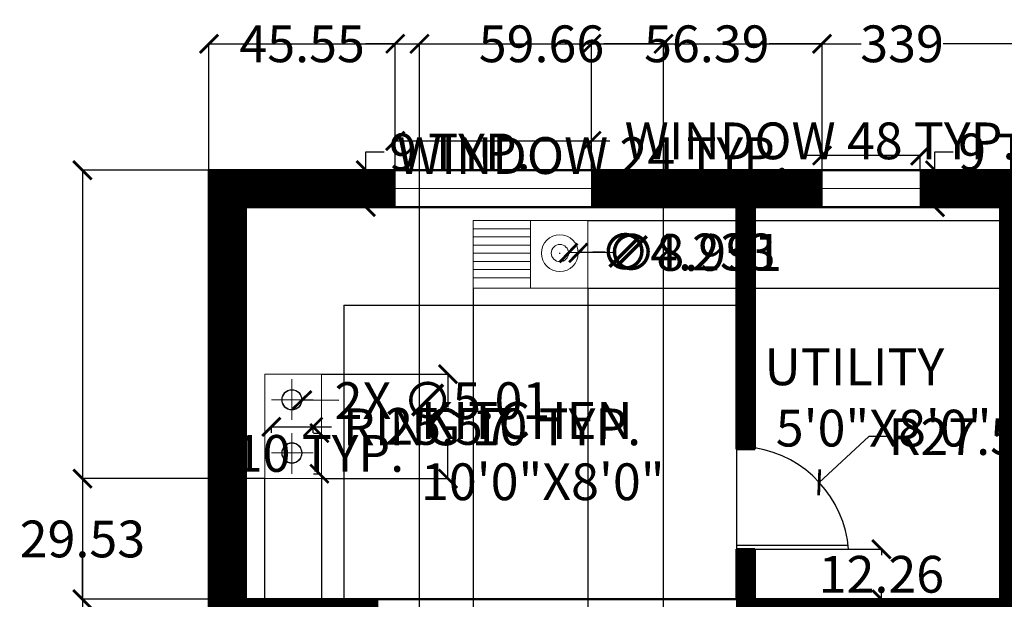
# Model space of a CAD drawing. Units: inches. Extents: x 91 to 526, y 242 to 861.
# Tile 4 of 5: x 91 to 332, y 719 to 861. Entities that reach past the tile are written whole.
import ezdxf

# ---------------------------------------------------------------- set-up
doc = ezdxf.new("R2010")
doc.units = ezdxf.units.IN
doc.header["$MEASUREMENT"] = 0
for name, color, linetype, lineweight in [('A-ANNO-DIMS', 2, 'Continuous', 18), ('A-AREA-IDEN', 7, 'Continuous', 18), ('A-DOOR', 3, 'Continuous', 25), ('A-EQPM', 8, 'Continuous', 18), ('A-FLOR-CASE', 8, 'Continuous', 25), ('A-FLOR-FIXT', 8, 'Continuous', 18), ('A-GLAZ', 4, 'Continuous', 18), ('A-WALL', 7, 'Continuous', 50), ('A-WALL-PATT', 252, 'Continuous', 13)]:
    doc.layers.add(name, color=color, linetype=linetype, lineweight=lineweight)
doc.styles.get("Standard").update_dxf_attribs({"font": 'arial.ttf'})
doc.dimstyles.get("Standard").update_dxf_attribs({"dimtxt": 9, "dimasz": 4.5, "dimexe": 0.18, "dimexo": 0.0625, "dimgap": 0.09, "dimtad": 0, "dimtih": 1, "dimtoh": 1, "dimdec": 1, "dimzin": 0, "dimdsep": 46, "dimlunit": 4, "dimtxsty": 'Standard', "dimblk": 'ARCHTICK', "dimcen": 0.09, "dimadec": 0, "dimazin": 0, "dimtfac": 1, "dimtdec": 1, "dimtofl": 0, "dimtmove": 0, "dimatfit": 3, "dimfxl": 1, "dimtolj": 1, "dimtzin": 0, "dimarcsym": 0})

# ---------------------------------------------------------------- blocks, each defined once
blk = doc.blocks.new('WIN-48')
for p, q in [((0, 9), (48, 9)), ((0, 0), (0, 9)), ((48, 9), (48, 0)), ((0, 4.5), (48, 4.5)), ((48, 0), (0, 0))]:
    blk.add_line(p, q)
blk = doc.blocks.new('WIN-24')
for p, q in [((0, 24), (9, 24)), ((0, 0), (0, 24)), ((4.5, 0), (4.5, 24)), ((9, 24), (9, 0)), ((0, 0), (9, 0))]:
    blk.add_line(p, q)
blk = doc.blocks.new('COOKTOP-BURNER')
for q in [(5.01, 9.95), (0, 4.87), (5.01, 0), (10.22, 4.87)]:
    blk.add_line((5.01, 4.87), q)
for radius in [2.5, 2.4]:
    blk.add_circle((5.01, 4.87), radius)
blk = doc.blocks.new('_ArchTick')
at = {"color": 0, "linetype": 'ByBlock', "const_width": 0.15}
blk.add_lwpolyline([(-0.5, -0.5), (0.5, 0.5)], dxfattribs=at)
blk = doc.blocks.new('*D7')
at = {"layer": 'A-ANNO-DIMS', "color": 0, "lineweight": -2, "transparency": 16777216}
for p, q in [((182.71, 823.73), (182.71, 831.05)), ((182.71, 830.87), (230.71, 830.87)), ((230.71, 823.73), (230.71, 831.05)), ((230.71, 830.87), (235.21, 830.87))]:
    blk.add_line(p, q, dxfattribs=at)
at = {"layer": 'Defpoints', "color": 0, "transparency": 16777216}
for p in [(230.71, 830.87), (182.71, 823.67), (230.71, 823.67)]:
    blk.add_point(p, dxfattribs=at)
at = {"layer": 'A-ANNO-DIMS', "color": 0, "lineweight": -2, "transparency": 16777216, "xscale": 4.5, "yscale": 4.5, "zscale": 4.5, "rotation": 180}
blk.add_blockref('_ArchTick', (182.71, 830.87), dxfattribs=at)
at = {"layer": 'A-ANNO-DIMS', "color": 0, "lineweight": -2, "transparency": 16777216, "xscale": 4.5, "yscale": 4.5, "zscale": 4.5}
blk.add_blockref('_ArchTick', (230.71, 830.87), dxfattribs=at)
at = {"layer": 'A-ANNO-DIMS', "color": 0, "transparency": 16777216, "insert": (286.72, 830.87), "char_height": 9, "attachment_point": 5}
blk.add_mtext('\\A1;WINDOW 48 TYP.', dxfattribs=at)
blk = doc.blocks.new('*D8')
at = {"layer": 'A-ANNO-DIMS', "color": 0, "lineweight": -2, "transparency": 16777216}
for p, q in [((175.51, 823.67), (175.51, 828.17)), ((175.51, 828.17), (180.01, 828.17)), ((182.65, 823.67), (175.33, 823.67)), ((175.51, 814.67), (175.51, 823.67)), ((182.65, 814.67), (175.33, 814.67))]:
    blk.add_line(p, q, dxfattribs=at)
at = {"layer": 'Defpoints', "color": 0, "transparency": 16777216}
for p in [(175.51, 823.67), (182.71, 823.67), (182.71, 814.67)]:
    blk.add_point(p, dxfattribs=at)
at = {"layer": 'A-ANNO-DIMS', "color": 0, "lineweight": -2, "transparency": 16777216, "xscale": 4.5, "yscale": 4.5, "zscale": 4.5}
for p, rotation in [((175.51, 823.67), 90), ((175.51, 814.67), 270)]:
    blk.add_blockref('_ArchTick', p, dxfattribs=dict(at, rotation=rotation))
at = {"layer": 'A-ANNO-DIMS', "color": 0, "transparency": 16777216, "insert": (198.51, 828.17), "char_height": 9, "attachment_point": 5}
blk.add_mtext('\\A1;9 TYP.', dxfattribs=at)
blk = doc.blocks.new('*D9')
at = {"layer": 'A-ANNO-DIMS', "color": 0, "lineweight": -2, "transparency": 16777216}
for p, q in [((287.1, 827.27), (282.6, 827.27)), ((287.1, 823.73), (287.1, 827.45)), ((311.1, 827.27), (287.1, 827.27)), ((311.1, 823.73), (311.1, 827.45))]:
    blk.add_line(p, q, dxfattribs=at)
at = {"layer": 'Defpoints', "color": 0, "transparency": 16777216}
for p in [(287.1, 827.27), (287.1, 823.67), (311.1, 823.67)]:
    blk.add_point(p, dxfattribs=at)
at = {"layer": 'A-ANNO-DIMS', "color": 0, "lineweight": -2, "transparency": 16777216, "xscale": 4.5, "yscale": 4.5, "zscale": 4.5, "rotation": 180}
blk.add_blockref('_ArchTick', (287.1, 827.27), dxfattribs=at)
at = {"layer": 'A-ANNO-DIMS', "color": 0, "lineweight": -2, "transparency": 16777216, "xscale": 4.5, "yscale": 4.5, "zscale": 4.5}
blk.add_blockref('_ArchTick', (311.1, 827.27), dxfattribs=at)
at = {"layer": 'A-ANNO-DIMS', "color": 0, "transparency": 16777216, "insert": (231.09, 827.27), "char_height": 9, "attachment_point": 5}
blk.add_mtext('\\A1;WINDOW 24 TYP.', dxfattribs=at)
blk = doc.blocks.new('*D10')
at = {"layer": 'A-ANNO-DIMS', "color": 0, "lineweight": -2, "transparency": 16777216}
for p, q in [((314.7, 823.67), (314.7, 828.17)), ((314.7, 828.17), (319.2, 828.17)), ((311.17, 823.67), (314.88, 823.67)), ((314.7, 814.67), (314.7, 823.67)), ((311.17, 814.67), (314.88, 814.67))]:
    blk.add_line(p, q, dxfattribs=at)
at = {"layer": 'Defpoints', "color": 0, "transparency": 16777216}
for p in [(311.1, 823.67), (314.7, 823.67), (311.1, 814.67)]:
    blk.add_point(p, dxfattribs=at)
at = {"layer": 'A-ANNO-DIMS', "color": 0, "lineweight": -2, "transparency": 16777216, "xscale": 4.5, "yscale": 4.5, "zscale": 4.5}
for p, rotation in [((314.7, 823.67), 90), ((314.7, 814.67), 270)]:
    blk.add_blockref('_ArchTick', p, dxfattribs=dict(at, rotation=rotation))
at = {"layer": 'A-ANNO-DIMS', "color": 0, "transparency": 16777216, "insert": (337.7, 828.17), "char_height": 9, "attachment_point": 5}
blk.add_mtext('\\A1;9 TYP.', dxfattribs=at)
blk = doc.blocks.new('*D15')
at = {"layer": 'A-ANNO-DIMS', "color": 0, "lineweight": -2, "transparency": 16777216}
for p, q in [((152.43, 759.41), (152.43, 761.06)), ((162.65, 759.41), (162.65, 761.06)), ((152.43, 760.88), (162.65, 760.88)), ((162.65, 760.88), (167.15, 760.88))]:
    blk.add_line(p, q, dxfattribs=at)
at = {"layer": 'Defpoints', "color": 0, "transparency": 16777216}
for p in [(152.43, 759.35), (162.65, 760.88), (162.65, 759.35)]:
    blk.add_point(p, dxfattribs=at)
at = {"layer": 'A-ANNO-DIMS', "color": 0, "lineweight": -2, "transparency": 16777216, "xscale": 4.5, "yscale": 4.5, "zscale": 4.5, "rotation": 180}
blk.add_blockref('_ArchTick', (152.43, 760.88), dxfattribs=at)
at = {"layer": 'A-ANNO-DIMS', "color": 0, "lineweight": -2, "transparency": 16777216, "xscale": 4.5, "yscale": 4.5, "zscale": 4.5}
blk.add_blockref('_ArchTick', (162.65, 760.88), dxfattribs=at)
at = {"layer": 'A-ANNO-DIMS', "color": 0, "transparency": 16777216, "insert": (206.38, 760.88), "char_height": 9, "attachment_point": 5}
blk.add_mtext('\\A1;RING 10 TYP.', dxfattribs=at)
blk = doc.blocks.new('*D16')
at = {"layer": 'A-ANNO-DIMS', "color": 0, "lineweight": -2, "transparency": 16777216}
for p, q in [((162.71, 759.35), (164.36, 759.35)), ((164.18, 759.35), (164.18, 759.06)), ((162.71, 749.4), (164.36, 749.4)), ((164.18, 749.4), (164.18, 749.69))]:
    blk.add_line(p, q, dxfattribs=at)
at = {"layer": 'Defpoints', "color": 0, "transparency": 16777216}
for p in [(162.65, 759.35), (162.65, 749.4), (164.18, 749.4)]:
    blk.add_point(p, dxfattribs=at)
at = {"layer": 'A-ANNO-DIMS', "color": 0, "lineweight": -2, "transparency": 16777216, "xscale": 4.5, "yscale": 4.5, "zscale": 4.5}
for p, rotation in [((164.18, 759.35), 90), ((164.18, 749.4), 270)]:
    blk.add_blockref('_ArchTick', p, dxfattribs=dict(at, rotation=rotation))
at = {"layer": 'A-ANNO-DIMS', "color": 0, "transparency": 16777216, "insert": (164.18, 754.38), "char_height": 9, "attachment_point": 5}
blk.add_mtext('\\A1;10 TYP.', dxfattribs=at)
blk = doc.blocks.new('*D17')
at = {"layer": 'A-ANNO-DIMS', "color": 0, "lineweight": -2, "transparency": 16777216}
for p, q in [((137.16, 823.73), (137.16, 854.8)), ((137.16, 854.62), (296.62, 854.62)), ((476.16, 854.62), (316.7, 854.62)), ((476.16, 823.73), (476.16, 854.8))]:
    blk.add_line(p, q, dxfattribs=at)
at = {"layer": 'Defpoints', "color": 0, "transparency": 16777216}
for p in [(476.16, 854.62), (137.16, 823.67), (476.16, 823.67)]:
    blk.add_point(p, dxfattribs=at)
at = {"layer": 'A-ANNO-DIMS', "color": 0, "lineweight": -2, "transparency": 16777216, "xscale": 4.5, "yscale": 4.5, "zscale": 4.5, "rotation": 180}
blk.add_blockref('_ArchTick', (137.16, 854.62), dxfattribs=at)
at = {"layer": 'A-ANNO-DIMS', "color": 0, "lineweight": -2, "transparency": 16777216, "xscale": 4.5, "yscale": 4.5, "zscale": 4.5}
blk.add_blockref('_ArchTick', (476.16, 854.62), dxfattribs=at)
at = {"layer": 'A-ANNO-DIMS', "color": 0, "transparency": 16777216, "insert": (306.66, 854.62), "char_height": 9, "attachment_point": 5}
blk.add_mtext('\\A1;339', dxfattribs=at)
blk = doc.blocks.new('*D18')
at = {"layer": 'A-ANNO-DIMS', "color": 0, "lineweight": -2, "transparency": 16777216}
for p, q in [((137.1, 823.67), (106.03, 823.67)), ((106.21, 823.67), (106.21, 570.36)), ((106.21, 307.67), (106.21, 560.99)), ((137.1, 307.67), (106.03, 307.67))]:
    blk.add_line(p, q, dxfattribs=at)
at = {"layer": 'Defpoints', "color": 0, "transparency": 16777216}
for p in [(106.21, 823.67), (137.16, 823.67), (137.16, 307.67)]:
    blk.add_point(p, dxfattribs=at)
at = {"layer": 'A-ANNO-DIMS', "color": 0, "lineweight": -2, "transparency": 16777216, "xscale": 4.5, "yscale": 4.5, "zscale": 4.5}
for p, rotation in [((106.21, 823.67), 90), ((106.21, 307.67), 270)]:
    blk.add_blockref('_ArchTick', p, dxfattribs=dict(at, rotation=rotation))
at = {"layer": 'A-ANNO-DIMS', "color": 0, "transparency": 16777216, "insert": (106.21, 565.67), "char_height": 9, "attachment_point": 5}
blk.add_mtext('\\A1;516', dxfattribs=at)
blk = doc.blocks.new('*D19')
at = {"layer": 'A-ANNO-DIMS', "color": 0, "lineweight": -2, "transparency": 16777216}
for p, q in [((137.16, 823.73), (137.16, 854.8)), ((137.16, 854.62), (144.45, 854.62)), ((182.71, 854.62), (175.43, 854.62)), ((182.71, 823.73), (182.71, 854.8))]:
    blk.add_line(p, q, dxfattribs=at)
at = {"layer": 'Defpoints', "color": 0, "transparency": 16777216}
for p in [(182.71, 854.62), (137.16, 823.67), (182.71, 823.67)]:
    blk.add_point(p, dxfattribs=at)
at = {"layer": 'A-ANNO-DIMS', "color": 0, "lineweight": -2, "transparency": 16777216, "xscale": 4.5, "yscale": 4.5, "zscale": 4.5, "rotation": 180}
blk.add_blockref('_ArchTick', (137.16, 854.62), dxfattribs=at)
at = {"layer": 'A-ANNO-DIMS', "color": 0, "lineweight": -2, "transparency": 16777216, "xscale": 4.5, "yscale": 4.5, "zscale": 4.5}
blk.add_blockref('_ArchTick', (182.71, 854.62), dxfattribs=at)
at = {"layer": 'A-ANNO-DIMS', "color": 0, "transparency": 16777216, "insert": (159.94, 854.62), "char_height": 9, "attachment_point": 5}
blk.add_mtext('\\A1;45.55', dxfattribs=at)
blk = doc.blocks.new('*D20')
at = {"layer": 'A-ANNO-DIMS', "color": 0, "lineweight": -2, "transparency": 16777216}
for p, q in [((230.71, 823.73), (230.71, 854.8)), ((230.71, 854.62), (243.62, 854.62)), ((287.1, 854.62), (274.19, 854.62)), ((287.1, 823.73), (287.1, 854.8))]:
    blk.add_line(p, q, dxfattribs=at)
at = {"layer": 'Defpoints', "color": 0, "transparency": 16777216}
for p in [(287.1, 854.62), (230.71, 823.67), (287.1, 823.67)]:
    blk.add_point(p, dxfattribs=at)
at = {"layer": 'A-ANNO-DIMS', "color": 0, "lineweight": -2, "transparency": 16777216, "xscale": 4.5, "yscale": 4.5, "zscale": 4.5, "rotation": 180}
blk.add_blockref('_ArchTick', (230.71, 854.62), dxfattribs=at)
at = {"layer": 'A-ANNO-DIMS', "color": 0, "lineweight": -2, "transparency": 16777216, "xscale": 4.5, "yscale": 4.5, "zscale": 4.5}
blk.add_blockref('_ArchTick', (287.1, 854.62), dxfattribs=at)
at = {"layer": 'A-ANNO-DIMS', "color": 0, "transparency": 16777216, "insert": (258.91, 854.62), "char_height": 9, "attachment_point": 5}
blk.add_mtext('\\A1;56.39', dxfattribs=at)
blk = doc.blocks.new('*D39')
at = {"layer": 'A-ANNO-DIMS', "color": 0, "lineweight": -2, "transparency": 16777216}
for p, q in [((201.78, 794.78), (201.78, 276.54)), ((229.79, 794.78), (229.79, 276.54)), ((201.78, 276.72), (229.79, 276.72)), ((229.79, 276.72), (234.29, 276.72))]:
    blk.add_line(p, q, dxfattribs=at)
at = {"layer": 'Defpoints', "color": 0, "transparency": 16777216}
for p in [(201.78, 794.84), (229.79, 794.84), (229.79, 276.72)]:
    blk.add_point(p, dxfattribs=at)
at = {"layer": 'A-ANNO-DIMS', "color": 0, "lineweight": -2, "transparency": 16777216, "xscale": 4.5, "yscale": 4.5, "zscale": 4.5, "rotation": 180}
blk.add_blockref('_ArchTick', (201.78, 276.72), dxfattribs=at)
at = {"layer": 'A-ANNO-DIMS', "color": 0, "lineweight": -2, "transparency": 16777216, "xscale": 4.5, "yscale": 4.5, "zscale": 4.5}
blk.add_blockref('_ArchTick', (229.79, 276.72), dxfattribs=at)
at = {"layer": 'A-ANNO-DIMS', "color": 0, "transparency": 16777216, "insert": (248.77, 276.72), "char_height": 9, "attachment_point": 5}
blk.add_mtext('\\A1;28.01', dxfattribs=at)
blk = doc.blocks.new('*D40')
at = {"layer": 'A-ANNO-DIMS', "color": 0, "lineweight": -2, "transparency": 16777216}
for p, q in [((229.85, 811.37), (507.29, 811.37)), ((507.11, 811.37), (507.11, 807.79)), ((507.11, 794.84), (507.11, 798.42)), ((229.85, 794.84), (507.29, 794.84))]:
    blk.add_line(p, q, dxfattribs=at)
at = {"layer": 'Defpoints', "color": 0, "transparency": 16777216}
for p in [(229.79, 811.37), (229.79, 794.84), (507.11, 794.84)]:
    blk.add_point(p, dxfattribs=at)
at = {"layer": 'A-ANNO-DIMS', "color": 0, "lineweight": -2, "transparency": 16777216, "xscale": 4.5, "yscale": 4.5, "zscale": 4.5}
for p, rotation in [((507.11, 811.37), 90), ((507.11, 794.84), 270)]:
    blk.add_blockref('_ArchTick', p, dxfattribs=dict(at, rotation=rotation))
at = {"layer": 'A-ANNO-DIMS', "color": 0, "transparency": 16777216, "insert": (507.11, 803.1), "char_height": 9, "attachment_point": 5}
blk.add_mtext('\\A1;16.528', dxfattribs=at)
blk = doc.blocks.new('*D41')
at = {"layer": 'A-ANNO-DIMS', "color": 0, "lineweight": -2, "transparency": 16777216}
for p, q in [((150.78, 748.14), (150.78, 276.54)), ((164.66, 748.14), (164.66, 276.54)), ((150.78, 276.72), (164.66, 276.72)), ((164.66, 276.72), (169.16, 276.72))]:
    blk.add_line(p, q, dxfattribs=at)
at = {"layer": 'Defpoints', "color": 0, "transparency": 16777216}
for p in [(150.78, 748.2), (164.66, 748.2), (164.66, 276.72)]:
    blk.add_point(p, dxfattribs=at)
at = {"layer": 'A-ANNO-DIMS', "color": 0, "lineweight": -2, "transparency": 16777216, "xscale": 4.5, "yscale": 4.5, "zscale": 4.5, "rotation": 180}
blk.add_blockref('_ArchTick', (150.78, 276.72), dxfattribs=at)
at = {"layer": 'A-ANNO-DIMS', "color": 0, "lineweight": -2, "transparency": 16777216, "xscale": 4.5, "yscale": 4.5, "zscale": 4.5}
blk.add_blockref('_ArchTick', (164.66, 276.72), dxfattribs=at)
at = {"layer": 'A-ANNO-DIMS', "color": 0, "transparency": 16777216, "insert": (184.01, 276.72), "char_height": 9, "attachment_point": 5}
blk.add_mtext('\\A1;13.87', dxfattribs=at)
blk = doc.blocks.new('*D42')
at = {"layer": 'A-ANNO-DIMS', "color": 0, "lineweight": -2, "transparency": 16777216}
for p, q in [((164.72, 773.77), (195.79, 773.77)), ((195.61, 773.77), (195.61, 765.67)), ((195.61, 748.2), (195.61, 756.3)), ((164.72, 748.2), (195.79, 748.2))]:
    blk.add_line(p, q, dxfattribs=at)
at = {"layer": 'Defpoints', "color": 0, "transparency": 16777216}
for p in [(164.66, 773.77), (164.66, 748.2), (195.61, 748.2)]:
    blk.add_point(p, dxfattribs=at)
at = {"layer": 'A-ANNO-DIMS', "color": 0, "lineweight": -2, "transparency": 16777216, "xscale": 4.5, "yscale": 4.5, "zscale": 4.5}
for p, rotation in [((195.61, 773.77), 90), ((195.61, 748.2), 270)]:
    blk.add_blockref('_ArchTick', p, dxfattribs=dict(at, rotation=rotation))
at = {"layer": 'A-ANNO-DIMS', "color": 0, "transparency": 16777216, "insert": (195.61, 760.99), "char_height": 9, "attachment_point": 5}
blk.add_mtext('\\A1;25.57', dxfattribs=at)
blk = doc.blocks.new('*D43')
at = {"layer": 'A-ANNO-DIMS', "color": 0, "lineweight": -2, "transparency": 16777216}
for p, q in [((150.72, 748.2), (106.03, 748.2)), ((106.21, 748.2), (106.21, 738.12)), ((106.21, 718.67), (106.21, 728.75)), ((146.1, 718.67), (106.03, 718.67))]:
    blk.add_line(p, q, dxfattribs=at)
at = {"layer": 'Defpoints', "color": 0, "transparency": 16777216}
for p in [(106.21, 748.2), (150.78, 748.2), (146.16, 718.67)]:
    blk.add_point(p, dxfattribs=at)
at = {"layer": 'A-ANNO-DIMS', "color": 0, "lineweight": -2, "transparency": 16777216, "xscale": 4.5, "yscale": 4.5, "zscale": 4.5}
for p, rotation in [((106.21, 748.2), 90), ((106.21, 718.67), 270)]:
    blk.add_blockref('_ArchTick', p, dxfattribs=dict(at, rotation=rotation))
at = {"layer": 'A-ANNO-DIMS', "color": 0, "transparency": 16777216, "insert": (106.21, 733.44), "char_height": 9, "attachment_point": 5}
blk.add_mtext('\\A1;29.53', dxfattribs=at)
blk = doc.blocks.new('*D44')
at = {"layer": 'A-ANNO-DIMS', "color": 0, "lineweight": -2, "transparency": 16777216}
for p, q in [((201.78, 794.78), (201.78, 276.54)), ((170.16, 790.61), (170.16, 276.54)), ((170.16, 276.72), (170.74, 276.72)), ((201.78, 276.72), (201.2, 276.72))]:
    blk.add_line(p, q, dxfattribs=at)
at = {"layer": 'Defpoints', "color": 0, "transparency": 16777216}
for p in [(201.78, 794.84), (170.16, 790.67), (201.78, 276.72)]:
    blk.add_point(p, dxfattribs=at)
at = {"layer": 'A-ANNO-DIMS', "color": 0, "lineweight": -2, "transparency": 16777216, "xscale": 4.5, "yscale": 4.5, "zscale": 4.5, "rotation": 180}
blk.add_blockref('_ArchTick', (170.16, 276.72), dxfattribs=at)
at = {"layer": 'A-ANNO-DIMS', "color": 0, "lineweight": -2, "transparency": 16777216, "xscale": 4.5, "yscale": 4.5, "zscale": 4.5}
blk.add_blockref('_ArchTick', (201.78, 276.72), dxfattribs=at)
at = {"layer": 'A-ANNO-DIMS', "color": 0, "transparency": 16777216, "insert": (185.97, 276.72), "char_height": 9, "attachment_point": 5}
blk.add_mtext('\\A1;31.62', dxfattribs=at)
blk = doc.blocks.new('*D45')
at = {"layer": 'A-ANNO-DIMS', "color": 0, "lineweight": -2, "transparency": 16777216}
for p, q in [((188.65, 668.08), (188.65, 854.8)), ((188.65, 854.62), (203.21, 854.62)), ((248.32, 854.62), (233.76, 854.62)), ((248.32, 668.08), (248.32, 854.8))]:
    blk.add_line(p, q, dxfattribs=at)
at = {"layer": 'Defpoints', "color": 0, "transparency": 16777216}
for p in [(248.32, 854.62), (188.65, 668.02), (248.32, 668.02)]:
    blk.add_point(p, dxfattribs=at)
at = {"layer": 'A-ANNO-DIMS', "color": 0, "lineweight": -2, "transparency": 16777216, "xscale": 4.5, "yscale": 4.5, "zscale": 4.5, "rotation": 180}
blk.add_blockref('_ArchTick', (188.65, 854.62), dxfattribs=at)
at = {"layer": 'A-ANNO-DIMS', "color": 0, "lineweight": -2, "transparency": 16777216, "xscale": 4.5, "yscale": 4.5, "zscale": 4.5}
blk.add_blockref('_ArchTick', (248.32, 854.62), dxfattribs=at)
at = {"layer": 'A-ANNO-DIMS', "color": 0, "transparency": 16777216, "insert": (218.48, 854.62), "char_height": 9, "attachment_point": 5}
blk.add_mtext('\\A1;59.66', dxfattribs=at)
blk = doc.blocks.new('*D54')
at = {"layer": 'A-ANNO-DIMS', "color": 0, "lineweight": -2, "transparency": 16777216}
for p, q in [((270.72, 730.93), (301.79, 730.93)), ((301.61, 730.93), (301.61, 729.49)), ((301.61, 718.67), (301.61, 720.12)), ((270.72, 718.67), (301.79, 718.67))]:
    blk.add_line(p, q, dxfattribs=at)
at = {"layer": 'Defpoints', "color": 0, "transparency": 16777216}
for p in [(270.66, 730.93), (270.66, 718.67), (301.61, 718.67)]:
    blk.add_point(p, dxfattribs=at)
at = {"layer": 'A-ANNO-DIMS', "color": 0, "lineweight": -2, "transparency": 16777216, "xscale": 4.5, "yscale": 4.5, "zscale": 4.5}
for p, rotation in [((301.61, 730.93), 90), ((301.61, 718.67), 270)]:
    blk.add_blockref('_ArchTick', p, dxfattribs=dict(at, rotation=rotation))
at = {"layer": 'A-ANNO-DIMS', "color": 0, "transparency": 16777216, "insert": (301.61, 724.8), "char_height": 9, "attachment_point": 5}
blk.add_mtext('\\A1;12.26', dxfattribs=at)
blk = doc.blocks.new('*D56')
at = {"layer": 'A-ANNO-DIMS', "color": 0, "lineweight": -2, "transparency": 16777216}
for p, q in [((222.89, 803.4), (223.07, 803.4)), ((222.98, 803.31), (222.98, 803.49)), ((236.47, 803.56), (227.47, 803.45))]:
    blk.add_line(p, q, dxfattribs=at)
at = {"layer": 'Defpoints', "color": 0, "transparency": 16777216}
for p in [(218.48, 803.34), (227.47, 803.45)]:
    blk.add_point(p, dxfattribs=at)
at = {"layer": 'A-ANNO-DIMS', "color": 0, "lineweight": -2, "transparency": 16777216, "xscale": 4.5, "yscale": 4.5, "zscale": 4.5, "rotation": 180.6930424715323}
blk.add_blockref('_ArchTick', (227.47, 803.45), dxfattribs=at)
at = {"layer": 'A-ANNO-DIMS', "color": 0, "transparency": 16777216, "insert": (255.78, 803.56), "char_height": 9, "attachment_point": 5}
blk.add_mtext('\\A1;∅8.991', dxfattribs=at)
blk = doc.blocks.new('*D57')
at = {"layer": 'A-ANNO-DIMS', "color": 0, "lineweight": -2, "transparency": 16777216}
for p, q in [((222.89, 803.4), (223.07, 803.4)), ((222.98, 803.31), (222.98, 803.49)), ((234.09, 803.68), (225.09, 803.45))]:
    blk.add_line(p, q, dxfattribs=at)
at = {"layer": 'Defpoints', "color": 0, "transparency": 16777216}
for p in [(220.86, 803.34), (225.09, 803.45)]:
    blk.add_point(p, dxfattribs=at)
at = {"layer": 'A-ANNO-DIMS', "color": 0, "lineweight": -2, "transparency": 16777216, "xscale": 4.5, "yscale": 4.5, "zscale": 4.5, "rotation": 181.4766467824964}
blk.add_blockref('_ArchTick', (225.09, 803.45), dxfattribs=at)
at = {"layer": 'A-ANNO-DIMS', "color": 0, "transparency": 16777216, "insert": (254.26, 803.68), "char_height": 9, "attachment_point": 5}
blk.add_mtext('\\A1;∅4.233', dxfattribs=at)
blk = doc.blocks.new('*D58')
at = {"layer": 'A-ANNO-DIMS', "color": 0, "lineweight": -2, "transparency": 16777216}
for p, q in [((157.35, 767.49), (157.53, 767.49)), ((157.44, 767.4), (157.44, 767.58)), ((168.94, 767.29), (159.95, 767.45))]:
    blk.add_line(p, q, dxfattribs=at)
at = {"layer": 'Defpoints', "color": 0, "transparency": 16777216}
for p in [(154.94, 767.54), (159.95, 767.45)]:
    blk.add_point(p, dxfattribs=at)
at = {"layer": 'A-ANNO-DIMS', "color": 0, "lineweight": -2, "transparency": 16777216, "xscale": 4.5, "yscale": 4.5, "zscale": 4.5, "rotation": 178.9910099189205}
blk.add_blockref('_ArchTick', (159.95, 767.45), dxfattribs=at)
at = {"layer": 'A-ANNO-DIMS', "color": 0, "transparency": 16777216, "insert": (194.26, 767.29), "char_height": 9, "attachment_point": 5}
blk.add_mtext('\\A1;2X ∅5.01', dxfattribs=at)
blk = doc.blocks.new('*D63')
at = {"layer": 'A-ANNO-DIMS', "color": 0, "lineweight": -2, "transparency": 16777216}
for p, q in [((298.53, 758.5), (286.39, 747.29)), ((303.03, 758.5), (298.53, 758.5)), ((266.07, 728.61), (266.25, 728.61)), ((266.16, 728.52), (266.16, 728.7))]:
    blk.add_line(p, q, dxfattribs=at)
at = {"layer": 'Defpoints', "color": 0, "transparency": 16777216}
for p in [(286.39, 747.29), (266.16, 728.61)]:
    blk.add_point(p, dxfattribs=at)
at = {"layer": 'A-ANNO-DIMS', "color": 0, "lineweight": -2, "transparency": 16777216, "xscale": 4.5, "yscale": 4.5, "zscale": 4.5, "rotation": 222.7186024980729}
blk.add_blockref('_ArchTick', (286.39, 747.29), dxfattribs=at)
at = {"layer": 'A-ANNO-DIMS', "color": 0, "transparency": 16777216, "insert": (322.6, 758.5), "char_height": 9, "attachment_point": 5}
blk.add_mtext('\\A1;R27.54', dxfattribs=at)

msp = doc.modelspace()

# ---------------------------------------------------------------- hatches: boundary and pattern name
at = {"layer": 'A-WALL-PATT'}
h = msp.add_hatch(dxfattribs=at)
h.set_pattern_fill('ANSI31', color=256)
h.paths.add_polyline_path([(476.1605, 544.131), (467.1605, 544.131), (467.1605, 469.6714), (381.2784, 469.6714), (381.2784, 467.1295, -0.01443214), (381.4527, 465.1714), (467.1605, 465.1714), (467.1605, 417.4774), (476.1605, 417.4774)])
h.paths.add_polyline_path([(476.1605, 637.294), (467.1605, 637.294), (467.1605, 618.1714), (383.1605, 618.1714), (383.1605, 650.6481), (381.8098, 650.6481, -0.04281846), (378.6605, 650.378), (378.6605, 618.1714), (378.6605, 613.6714), (467.1605, 613.6714), (467.1605, 592.131), (476.1605, 592.131)])
h.paths.add_polyline_path([(476.1605, 699.6337), (467.1605, 699.6337), (467.1605, 682.6714), (378.6605, 682.6714), (367.8126, 682.6714), (367.8126, 678.1714), (378.6605, 678.1714), (378.6605, 668.8665), (383.1605, 668.8665), (383.1605, 678.1714), (467.1605, 678.1714), (467.1605, 661.294), (476.1605, 661.294)])
h.paths.add_polyline_path([(476.1605, 823.6714), (423.2305, 823.6714), (423.2305, 814.6714), (467.1605, 814.6714), (467.1605, 747.6337), (476.1605, 747.6337)])
h.paths.add_polyline_path([(375.2305, 823.6714), (311.1029, 823.6714), (311.1029, 814.6714), (330.6605, 814.6714), (330.6605, 682.6714), (335.1605, 682.6714), (335.1605, 814.6714), (375.2305, 814.6714)])
h.paths.add_polyline_path([(287.1029, 823.6714), (230.7133, 823.6714), (230.7133, 814.6714), (266.1605, 814.6714), (266.1605, 755.4247), (270.6605, 755.4247), (270.6605, 814.6714), (287.1029, 814.6714)])
h.paths.add_polyline_path([(182.7133, 823.6714), (137.1605, 823.6714), (137.1605, 675.6513), (146.1605, 675.6513), (146.1605, 714.1714), (178.4758, 714.1714), (178.4758, 718.6714), (146.1605, 718.6714), (146.1605, 814.6714), (182.7133, 814.6714)])
h.paths.add_polyline_path([(146.1605, 577.6714), (206.1605, 577.6714), (206.1605, 557.5953), (210.6605, 557.5953), (210.6605, 577.6714), (233.4933, 577.6714), (233.4933, 582.1714), (210.6605, 582.1714), (146.1605, 582.1714), (146.1605, 627.6513), (137.1605, 627.6513), (137.1605, 508.0167), (146.1605, 508.0167), (146.1605, 525.1714), (210.6605, 525.1714), (233.4933, 525.1714), (233.4933, 529.6714), (210.6605, 529.6714), (210.6605, 536.5826), (206.1605, 536.5826), (206.1605, 529.6714), (146.1605, 529.6714)])
h.paths.add_polyline_path([(146.1605, 460.0167), (137.1605, 460.0167), (137.1605, 360.2935), (146.1605, 360.2935), (146.1605, 376.6714), (210.6605, 376.6714), (213.2441, 376.6714, -0.02418169), (213.3544, 378.9513), (213.3544, 381.1714), (210.6605, 381.1714), (146.1605, 381.1714)])
h.paths.add_polyline_path([(146.1605, 336.2935), (137.1605, 336.2935), (137.1605, 307.6714), (146.1605, 307.6714), (177.3362, 307.6714), (177.3362, 316.6714), (146.1605, 316.6714)])
h.paths.add_polyline_path([(393.6086, 316.6714), (323.4726, 316.6714), (323.4726, 307.6714), (393.6086, 307.6714)])
h.paths.add_polyline_path([(256.39, 316.6714), (201.3362, 316.6714), (201.3362, 307.6714), (256.39, 307.6714)])
h.paths.add_polyline_path([(246.6605, 376.6714), (246.6605, 381.1714), (236.8559, 381.1714), (236.8559, 376.6714), (242.1605, 376.6714), (242.1605, 316.6714), (246.6605, 316.6714)])
h = msp.add_hatch(dxfattribs=at)
h.set_pattern_fill('ANSI31', color=256)
h.paths.add_polyline_path([(476.1605, 369.4774), (467.1605, 369.4774), (467.1605, 316.6714), (417.6086, 316.6714), (417.6086, 307.6714), (476.1605, 307.6714)])
h.paths.add_polyline_path([(330.6605, 718.6714), (270.6605, 718.6714), (270.6605, 730.9304), (266.1605, 730.9304), (266.1605, 718.6714), (266.1605, 714.1714), (270.6605, 714.1714), (330.6605, 714.1714)])

# ---------------------------------------------------------------- linework, layer by layer
at = {"layer": 'A-DOOR'}
for p, q in [((266.1605, 755.4247), (266.1605, 730.9304)), ((266.1605, 731.9304), (293.499, 731.9304)), ((266.1605, 730.9304), (266.1605, 730.9304)), ((266.1605, 730.9304), (293.6021, 730.9304))]:
    msp.add_line(p, q, dxfattribs=at)
msp.add_arc((266.1605, 728.6069), 27.5398, 4.839769, 80.595694, dxfattribs=at)
at = {"layer": 'A-EQPM'}
for p, q in [((150.7847, 773.7724), (164.6554, 773.7724)), ((150.7847, 748.2001), (150.7847, 773.7724)), ((164.6554, 773.7724), (164.6554, 748.2001)), ((164.6554, 748.2001), (150.7847, 748.2001))]:
    msp.add_line(p, q, dxfattribs=at)
at = {"layer": 'A-FLOR-CASE'}
for q in [(266.1605, 790.6714), (170.1605, 718.6714)]:
    msp.add_line((170.1605, 790.6714), q, dxfattribs=at)
at = {"layer": 'A-FLOR-FIXT'}
for p, q in [((201.7777, 811.367), (229.7885, 811.367)), ((201.7777, 794.8389), (201.7777, 811.367)), ((201.7777, 809.367), (215.7831, 809.367)), ((215.7831, 811.367), (215.7831, 794.8389)), ((229.7885, 811.367), (229.7885, 794.8389)), ((201.7777, 807.367), (215.7831, 807.367)), ((201.7777, 805.367), (215.7831, 805.367)), ((201.7777, 805.367), (215.7831, 805.367)), ((201.7777, 803.367), (215.7831, 803.367)), ((201.7777, 801.367), (215.7831, 801.367)), ((201.7777, 799.367), (215.7831, 799.367)), ((201.7777, 797.367), (215.7831, 797.367)), ((229.7885, 794.8389), (201.7777, 794.8389))]:
    msp.add_line(p, q, dxfattribs=at)
for radius in [4.4956, 2.1167]:
    msp.add_circle((222.9781, 803.3953), radius, dxfattribs=at)
at = {"layer": 'A-GLAZ'}
for p, q in [((178.4758, 718.6714), (178.4758, 714.1714)), ((266.1605, 718.6714), (266.1605, 714.1714))]:
    msp.add_line(p, q, dxfattribs=at)
at = {"layer": 'A-WALL'}
for p, q in [((137.1605, 823.6714), (137.1605, 307.6714)), ((137.1605, 823.6714), (476.1605, 823.6714)), ((146.1605, 814.6714), (146.1605, 718.6714)), ((146.1605, 814.6714), (266.1605, 814.6714)), ((266.1605, 814.6714), (266.1605, 755.4247)), ((270.6605, 814.6714), (270.6605, 755.4247)), ((270.6605, 814.6714), (330.6605, 814.6714)), ((330.6605, 814.6714), (330.6605, 682.6714)), ((266.1605, 755.4247), (270.6605, 755.4247)), ((266.1605, 730.9304), (270.6605, 730.9304)), ((266.1605, 730.9304), (266.1605, 718.6714)), ((270.6605, 730.9304), (270.6605, 718.6714)), ((146.1605, 718.6714), (266.1605, 718.6714)), ((270.6605, 718.6714), (330.6605, 718.6714))]:
    msp.add_line(p, q, dxfattribs=at)

# ---------------------------------------------------------------- block references
at = {"layer": 'A-EQPM'}
msp.add_blockref('COOKTOP-BURNER', (152.432, 762.621), dxfattribs=at)
at = {"layer": 'A-EQPM', "extrusion": (0, 0, -1), "zscale": -1, "rotation": 180}
msp.add_blockref('COOKTOP-BURNER', (-152.432, 759.3515), dxfattribs=at)
at = {"layer": 'A-GLAZ'}
msp.add_blockref('WIN-48', (182.713, 814.671), dxfattribs=at)
at = {"layer": 'A-GLAZ', "rotation": 89.99999999999989}
msp.add_blockref('WIN-24', (311.1034, 814.6719), dxfattribs=at)

# ---------------------------------------------------------------- texts
at = {"layer": 'A-AREA-IDEN', "char_height": 9, "attachment_point": 1}
for s, insert in [('  UTILITY\\P   5\'0"X8\'0"', (267.5236, 780.0703)), ('  KITCHEN\\P  10\'0"X8\'0"', (183.5059, 766.9463))]:
    msp.add_mtext_dynamic_manual_height_columns(s, width=356.121763, gutter_width=1, heights=[0], dxfattribs=dict(at, insert=insert))

# ---------------------------------------------------------------- dimensions: what is measured, and where the dimension line sits
at = {"layer": 'A-ANNO-DIMS'}
for base, p1, p2, override, picture, middle in [((476.1605, 854.6214), (137.1605, 823.6714), (476.1605, 823.6714), {"dimdec": 0, "dimlfac": 1, "dimrnd": 0, "dimzin": 0, "dimdsep": 46, "dimlunit": 2}, '*D17', (306.6605, 854.6214)), ((182.7133, 854.6214), (137.1605, 823.6714), (182.7133, 823.6714), {"dimdec": 2, "dimlfac": 1, "dimrnd": 0, "dimzin": 0, "dimdsep": 46, "dimlunit": 2}, '*D19', (159.9369, 854.6214)), ((248.3166, 854.6214), (188.6533, 668.0163), (248.3166, 668.0163), {"dimdec": 2, "dimlfac": 1, "dimrnd": 0, "dimzin": 0, "dimdsep": 46, "dimlunit": 2}, '*D45', (218.485, 854.6214)), ((287.1029, 854.6214), (230.7133, 823.6714), (287.1029, 823.6714), {"dimdec": 2, "dimlfac": 1, "dimrnd": 0, "dimzin": 0, "dimdsep": 46, "dimlunit": 2}, '*D20', (258.9081, 854.6214)), ((201.7777, 276.7214), (170.1605, 790.6714), (201.7777, 794.8389), {"dimdec": 2, "dimlfac": 1, "dimrnd": 0, "dimzin": 0, "dimdsep": 46, "dimlunit": 2}, '*D44', (185.9691, 276.7214)), ((229.7885, 276.7214), (201.7777, 794.8389), (229.7885, 794.8389), {"dimdec": 2, "dimlfac": 1, "dimrnd": 0, "dimzin": 0, "dimdsep": 46, "dimlunit": 2}, '*D39', (248.7718, 276.7214)), ((164.6554, 276.7214), (150.7847, 748.2001), (164.6554, 748.2001), {"dimdec": 2, "dimlfac": 1, "dimrnd": 0, "dimzin": 0, "dimdsep": 46, "dimlunit": 2}, '*D41', (184.007, 276.7214))]:
    dim = msp.add_linear_dim(base=base, p1=p1, p2=p2, dimstyle='Standard', override=override, dxfattribs=at)
    dim.commit()
    dim.dimension.update_dxf_attribs({"geometry": picture, "text_midpoint": middle})
for base, p1, p2, text, picture, middle in [((230.7133, 830.8714), (182.7133, 823.6714), (230.7133, 823.6714), 'WINDOW <> TYP.', '*D7', (286.7218, 830.8714)), ((162.6515, 760.8849), (152.4319, 759.3519), (162.6515, 759.3519), 'RING <> TYP.', '*D15', (206.3755, 760.8849))]:
    dim = msp.add_linear_dim(base=base, p1=p1, p2=p2, text=text, dimstyle='Standard', override={"dimdec": 0, "dimlfac": 1, "dimrnd": 0, "dimzin": 0, "dimdsep": 46, "dimlunit": 2}, dxfattribs=at)
    dim.commit()
    dim.dimension.update_dxf_attribs({"geometry": picture, "text_midpoint": middle})
for base, p1, p2, angle, text, picture, middle in [((287.1029, 827.2714), (311.1029, 823.6714), (287.1029, 823.6714), 180, 'WINDOW <> TYP.', '*D9', (231.0944, 827.2714)), ((175.5133, 823.6714), (182.7133, 814.6714), (182.7133, 823.6714), 90, '<> TYP.', '*D8', (198.5116, 828.1714)), ((314.7029, 823.6714), (311.1029, 814.6714), (311.1029, 823.6714), 90, '<> TYP.', '*D10', (337.7012, 828.1714)), ((164.1844, 749.4045), (162.6515, 759.3519), (162.6515, 749.4045), 270, '<> TYP.', '*D16', (164.1844, 754.3782))]:
    dim = msp.add_linear_dim(base=base, p1=p1, p2=p2, angle=angle, text=text, dimstyle='Standard', override={"dimdec": 0, "dimlfac": 1, "dimrnd": 0, "dimzin": 0, "dimdsep": 46, "dimlunit": 2}, dxfattribs=at)
    dim.commit()
    dim.dimension.update_dxf_attribs({"geometry": picture, "text_midpoint": middle})
for base, p1, p2, angle, override, picture, middle in [((106.2105, 823.6714), (137.1605, 307.6714), (137.1605, 823.6714), 90, {"dimdec": 0, "dimlfac": 1, "dimrnd": 0, "dimzin": 0, "dimdsep": 46, "dimlunit": 2}, '*D18', (106.2105, 565.6714)), ((507.1105, 794.8389), (229.7885, 811.367), (229.7885, 794.8389), 90, {"dimdec": 3, "dimlfac": 1, "dimrnd": 0, "dimzin": 0, "dimdsep": 46, "dimlunit": 2}, '*D40', (507.1105, 803.1029)), ((195.6054, 748.2001), (164.6554, 773.7724), (164.6554, 748.2001), 270, {"dimdec": 2, "dimlfac": 1, "dimrnd": 0, "dimzin": 0, "dimdsep": 46, "dimlunit": 2}, '*D42', (195.6054, 760.9863)), ((106.2105, 748.2001), (146.1605, 718.6714), (150.7847, 748.2001), 90, {"dimdec": 2, "dimlfac": 1, "dimrnd": 0, "dimzin": 0, "dimdsep": 46, "dimlunit": 2}, '*D43', (106.2105, 733.4358)), ((301.6105, 718.6714), (270.6605, 730.9304), (270.6605, 718.6714), 270, {"dimdec": 2, "dimlfac": 1, "dimrnd": 0, "dimzin": 0, "dimdsep": 46, "dimlunit": 2}, '*D54', (301.6105, 724.8009))]:
    dim = msp.add_linear_dim(base=base, p1=p1, p2=p2, angle=angle, dimstyle='Standard', override=override, dxfattribs=at)
    dim.commit()
    dim.dimension.update_dxf_attribs({"geometry": picture, "text_midpoint": middle})
for p1, p2, picture, middle in [((218.4828, 803.3409), (227.4734, 803.4497), '*D56', (236.4727, 803.5585)), ((220.8621, 803.3408), (225.094, 803.4498), '*D57', (234.091, 803.6818))]:
    dim = msp.add_diameter_dim_2p(p1=p1, p2=p2, dimstyle='Standard', override={"dimdec": 3, "dimlfac": 1, "dimrnd": 0, "dimzin": 0, "dimdsep": 46, "dimlunit": 2}, dxfattribs=at)
    dim.commit()
    dim.dimension.update_dxf_attribs({"geometry": picture, "text_midpoint": middle, "dimtype": 163})
dim = msp.add_diameter_dim_2p(p1=(154.9371, 767.5383), p2=(159.9459, 767.4501), text='2X <>', dimstyle='Standard', override={"dimdec": 2, "dimlfac": 1, "dimrnd": 0, "dimzin": 0, "dimdsep": 46, "dimlunit": 2}, dxfattribs=at)
dim.commit()
dim.dimension.update_dxf_attribs({"geometry": '*D58', "text_midpoint": (168.9445, 767.2916), "dimtype": 163})
dim = msp.add_radius_dim(center=(266.1605, 728.6069), mpoint=(286.3938, 747.2898), dimstyle='Standard', override={"dimdec": 2, "dimlfac": 1, "dimrnd": 0, "dimzin": 0, "dimdsep": 46, "dimlunit": 2}, dxfattribs=at)
dim.commit()
dim.dimension.update_dxf_attribs({"geometry": '*D63', "text_midpoint": (322.5972, 758.4996), "dimtype": 164})

doc.saveas('drawing.dxf')
